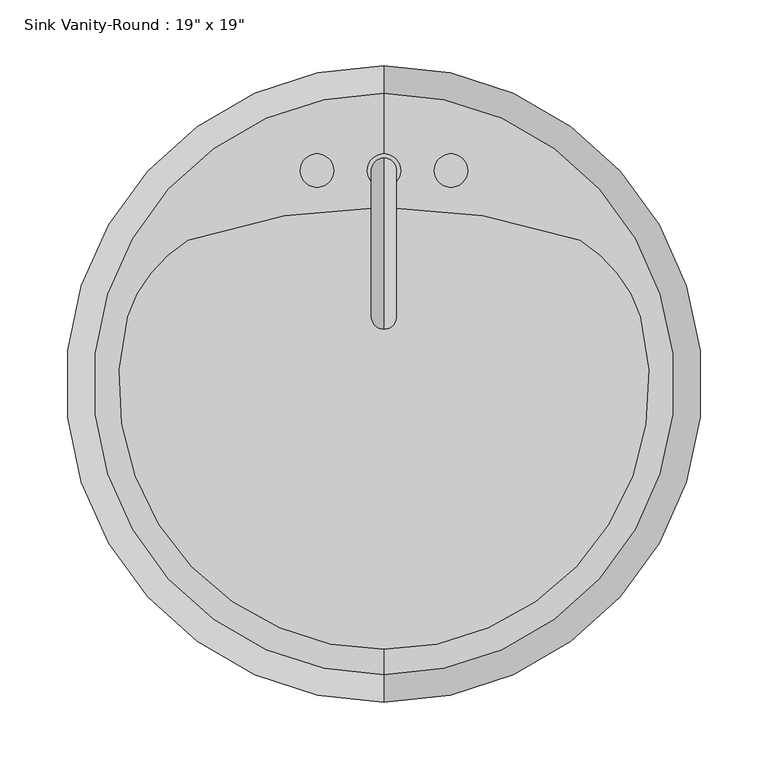
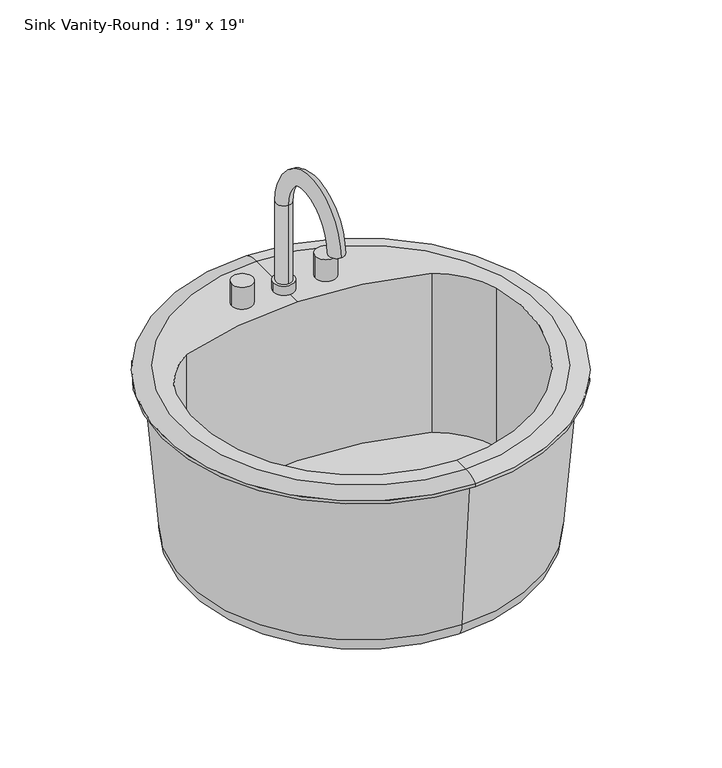
"""IFC4 building model written with IfcOpenShell, lengths in millimetres: flow terminal geometry."""

from ifc_helpers import new_model, si_unit, point, frame, frame_2d, origin, place, context, project, spatial, polyline, circle_curve, ellipse_curve, trimmed, segment, composite_curve, outline, extrude, source, transform, mapped, element, save
from ifc_brep_helpers import plane_surface, cylinder_surface, revolved_surface, advanced_brep


def flow_terminal_a43f4bde(model_context):
    return source(origin(), model_context, "Body", "SolidModel", [
        advanced_brep(
        [(96.6517406, -135.3870093, 796.925), (96.6517406, 305.7224463, 796.925), (96.6517406, 326.4677185, 791.36875), (96.6517406, -156.1322815, 791.36875), (96.6517406, -116.2405705, 796.925), (-98.1703414, 136.2525038, 796.925), (-52.1534933, 194.0861398, 796.925), (96.6517406, 219.2662048, 796.925), (245.4569744, 194.0861398, 796.925), (291.4738225, 136.2525038, 796.925), (96.6517406, -107.1264028, 571.5), (96.6517406, 277.4618398, 571.5), (96.6517406, 85.1677185, 571.5), (96.6517406, -127.6827361, 592.6842611), (96.6517406, 298.0181731, 592.6842611), (96.6517406, -144.2260315, 787.4), (96.6517406, 314.5614685, 787.4), (96.6517406, -156.1322815, 787.4), (96.6517406, 326.4677185, 787.4), (245.4569744, 194.0861398, 592.6842611), (-52.1534933, 194.0861398, 592.6842611), (-98.1703414, 136.2525038, 592.6842611), (291.4738225, 136.2525038, 592.6842611)],
        [
            (0, 1, circle_curve(frame((96.6517406, 85.1677185, 796.925), z_axis=(0.0, 0.0, -1.0), x_axis=(0.0, 1.0, 0.0)), 220.5547278)),
            (1, 2, circle_curve(frame((96.6517406, 309.4374616, 769.289434), z_axis=(-1.0, 0.0, 0.0), x_axis=(0.0, 1.0, 0.0)), 27.8841505)),
            (2, 3, circle_curve(frame((96.6517406, 85.1677185, 791.36875), z_axis=(0.0, 0.0, 1.0), x_axis=(0.0, 1.0, 0.0)), 241.3)),
            (3, 0, circle_curve(frame((96.6517406, -139.1020246, 769.289434), z_axis=(-1.0, 0.0, 0.0), x_axis=(0.0, -1.0, 0.0)), 27.8841505)),
            (1, 0, circle_curve(frame((96.6517406, 85.1677185, 796.925), z_axis=(0.0, 0.0, -1.0), x_axis=(0.0, 1.0, 0.0)), 220.5547278)),
            (3, 2, circle_curve(frame((96.6517406, 85.1677185, 791.36875), z_axis=(0.0, 0.0, 1.0), x_axis=(0.0, 1.0, 0.0)), 241.3)),
            (0, 4),
            (4, 5, circle_curve(frame((96.6517406, 85.1677185, 796.925), z_axis=(0.0, 0.0, -1.0), x_axis=(1.0, 0.0, 0.0)), 201.408289)),
            (5, 6, circle_curve(frame((1.3689689, 104.2755165, 796.925), z_axis=(0.0, 0.0, -1.0), x_axis=(1.0, 0.0, 0.0)), 104.5495194)),
            (6, 7, circle_curve(frame((96.6517406, -233.0168462, 796.925), z_axis=(0.0, 0.0, -1.0), x_axis=(1.0, 0.0, 0.0)), 452.283051)),
            (7, 1),
            (7, 8, circle_curve(frame((96.6517406, -233.0168462, 796.925), z_axis=(0.0, 0.0, -1.0), x_axis=(1.0, 0.0, 0.0)), 452.283051)),
            (8, 9, circle_curve(frame((191.9345122, 104.2755165, 796.925), z_axis=(0.0, 0.0, -1.0), x_axis=(1.0, 0.0, 0.0)), 104.5495194)),
            (9, 4, circle_curve(frame((96.6517406, 85.1677185, 796.925), z_axis=(0.0, 0.0, -1.0), x_axis=(1.0, 0.0, 0.0)), 201.408289)),
            (10, 11, circle_curve(frame((96.6517406, 85.1677185, 571.5), z_axis=(0.0, 0.0, -1.0), x_axis=(0.0, 1.0, 0.0)), 192.2941213)),
            (11, 12),
            (12, 10),
            (11, 10, circle_curve(frame((96.6517406, 85.1677185, 571.5), z_axis=(0.0, 0.0, -1.0), x_axis=(0.0, 1.0, 0.0)), 192.2941213)),
            (10, 13, circle_curve(frame((96.6517406, -107.1264028, 592.0656396), z_axis=(-1.0, 0.0, 0.0), x_axis=(0.0, -1.0, 0.0)), 20.5656396)),
            (13, 14, circle_curve(frame((96.6517406, 85.1677185, 592.6842611), z_axis=(0.0, 0.0, -1.0), x_axis=(0.0, 1.0, 0.0)), 212.8504546)),
            (14, 11, circle_curve(frame((96.6517406, 277.4618398, 592.0656396), z_axis=(-1.0, 0.0, 0.0), x_axis=(0.0, 1.0, 0.0)), 20.5656396)),
            (14, 13, circle_curve(frame((96.6517406, 85.1677185, 592.6842611), z_axis=(0.0, 0.0, -1.0), x_axis=(0.0, 1.0, 0.0)), 212.8504546)),
            (13, 15),
            (15, 16, circle_curve(frame((96.6517406, 85.1677185, 787.4), z_axis=(0.0, 0.0, -1.0), x_axis=(0.0, 1.0, 0.0)), 229.39375)),
            (16, 14),
            (16, 15, circle_curve(frame((96.6517406, 85.1677185, 787.4), z_axis=(0.0, 0.0, -1.0), x_axis=(0.0, 1.0, 0.0)), 229.39375)),
            (15, 17),
            (17, 18, circle_curve(frame((96.6517406, 85.1677185, 787.4), z_axis=(0.0, 0.0, -1.0), x_axis=(0.0, 1.0, 0.0)), 241.3)),
            (18, 16),
            (18, 17, circle_curve(frame((96.6517406, 85.1677185, 787.4), z_axis=(0.0, 0.0, -1.0), x_axis=(0.0, 1.0, 0.0)), 241.3)),
            (2, 18),
            (17, 3),
            (19, 20, circle_curve(frame((96.6517406, -233.0168462, 592.6842611), z_axis=(0.0, 0.0, 1.0), x_axis=(1.0, 0.0, 0.0)), 452.283051)),
            (20, 21, circle_curve(frame((1.3689689, 104.2755165, 592.6842611), z_axis=(0.0, 0.0, 1.0), x_axis=(1.0, 0.0, 0.0)), 104.5495194)),
            (21, 22, circle_curve(frame((96.6517406, 85.1677185, 592.6842611), z_axis=(0.0, 0.0, 1.0), x_axis=(1.0, 0.0, 0.0)), 201.408289)),
            (22, 19, circle_curve(frame((191.9345122, 104.2755165, 592.6842611), z_axis=(0.0, 0.0, 1.0), x_axis=(1.0, 0.0, 0.0)), 104.5495194)),
            (19, 8),
            (6, 20),
            (5, 21),
            (9, 22),
        ],
        [
            revolved_surface(trimmed(ellipse_curve(frame((96.6517406, 309.4374616, 769.289434), z_axis=(1.0, 0.0, 0.0), x_axis=(0.0, 1.0, 0.0)), 27.8841505, 27.8841505), [point((96.6517406, 326.4677185, 791.36875))], [point((96.6517406, 305.7224463, 796.925))], True, "CARTESIAN"), (96.6517406, 85.1677185, 796.925), (0.0, 0.0, 1.0)),
            plane_surface(frame((96.6517406, 85.1677185, 796.925), z_axis=(0.0, 0.0, 1.0), x_axis=(0.0, 1.0, 0.0))),
            plane_surface(frame((96.6517406, 85.1677185, 571.5), z_axis=(0.0, 0.0, -1.0), x_axis=(0.0, 1.0, 0.0))),
            revolved_surface(trimmed(ellipse_curve(frame((96.6517406, 277.4618398, 592.0656396), z_axis=(1.0, 0.0, 0.0), x_axis=(0.0, 1.0, 0.0)), 20.5656396, 20.5656396), [point((96.6517406, 277.4618398, 571.5))], [point((96.6517406, 298.0181731, 592.6842611))], True, "CARTESIAN"), (96.6517406, 85.1677185, 796.925), (0.0, 0.0, 1.0)),
            revolved_surface(polyline([(96.6517406, 298.0181731, 592.6842611), (96.6517406, 314.5614685, 787.4)]), (96.6517406, 85.1677185, 796.925), (0.0, 0.0, 1.0)),
            plane_surface(frame((96.6517406, 85.1677185, 787.4), z_axis=(0.0, 0.0, -1.0), x_axis=(0.0, 1.0, 0.0))),
            cylinder_surface(frame((96.6517406, 85.1677185, 796.925), z_axis=(0.0, 0.0, 1.0), x_axis=(0.0, 1.0, 0.0)), 241.3),
            plane_surface(frame((548.9347916, -233.0168462, 592.6842611), z_axis=(0.0, 0.0, 1.0), x_axis=(0.0, -1.0, 0.0))),
            revolved_surface(polyline([(548.9347916, -233.0168462, 796.925), (548.9347916, -233.0168462, 592.6842611)]), (96.6517406, -233.0168462, 592.6842611), (0.0, 0.0, 1.0)),
            revolved_surface(polyline([(105.91848829999999, 104.2755165, 796.925), (105.91848829999999, 104.2755165, 592.6842611)]), (1.3689689, 104.2755165, 592.6842611), (0.0, 0.0, 1.0)),
            revolved_surface(polyline([(298.0600296, 85.1677185, 796.925), (298.0600296, 85.1677185, 592.6842611)]), (96.6517406, 85.1677185, 592.6842611), (0.0, 0.0, 1.0)),
            revolved_surface(polyline([(296.4840316, 104.2755165, 796.925), (296.4840316, 104.2755165, 592.6842611)]), (191.9345122, 104.2755165, 592.6842611), (0.0, 0.0, 1.0)),
        ],
        [
            (0, [[1, 2, 3, 4]]),
            (0, [[-2, 5, -4, 6]]),
            (1, [[-1, 7, 8, 9, 10, 11]]),
            (1, [[-5, -11, 12, 13, 14, -7]]),
            (2, [[15, 16, 17]]),
            (2, [[-16, 18, -17]]),
            (3, [[-15, 19, 20, 21]]),
            (3, [[-18, -21, 22, -19]]),
            (4, [[-20, 23, 24, 25]]),
            (4, [[-22, -25, 26, -23]]),
            (5, [[-24, 27, 28, 29]]),
            (5, [[-26, -29, 30, -27]]),
            (6, [[-3, 31, -28, 32]]),
            (6, [[-6, -32, -30, -31]]),
            (7, [[33, 34, 35, 36]]),
            (8, [[-33, 37, -12, -10, 38]]),
            (9, [[-34, -38, -9, 39]]),
            (10, [[-35, -39, -8, -14, 40]]),
            (11, [[-36, -40, -13, -37]]),
        ],
    ),
        extrude(outline(composite_curve([segment(trimmed(circle_curve(frame_2d((96.6517406, 85.1677185)), 20.6375), [point((76.0142406, 85.1677185))], [point((117.2892406, 85.1677185))], False, "CARTESIAN"), True, "CONTINUOUS"), segment(trimmed(circle_curve(frame_2d((96.6517406, 85.1677185)), 20.6375), [point((117.2892406, 85.1677185))], [point((76.0142406, 85.1677185))], False, "CARTESIAN"), True, "CONTINUOUS")], self_intersect=False)), frame((0.0, 0.0, 571.5), z_axis=(0.0, 0.0, 1.0), x_axis=(1.0, 0.0, 0.0)), (0.0, 0.0, 1.0), 21.1842611),
        extrude(outline(composite_curve([segment(trimmed(circle_curve(frame_2d((147.4517406, 247.0927185)), 12.7), [point((134.7517406, 247.0927185))], [point((160.1517406, 247.0927185))], False, "CARTESIAN"), True, "CONTINUOUS"), segment(trimmed(circle_curve(frame_2d((147.4517406, 247.0927185)), 12.7), [point((160.1517406, 247.0927185))], [point((134.7517406, 247.0927185))], False, "CARTESIAN"), True, "CONTINUOUS")], self_intersect=False)), frame((0.0, 0.0, 796.925), z_axis=(0.0, 0.0, 1.0), x_axis=(1.0, 0.0, 0.0)), (0.0, 0.0, 1.0), 28.575),
        extrude(outline(composite_curve([segment(trimmed(circle_curve(frame_2d((45.8517406, 247.0927185)), 12.7), [point((33.1517406, 247.0927185))], [point((58.5517406, 247.0927185))], False, "CARTESIAN"), True, "CONTINUOUS"), segment(trimmed(circle_curve(frame_2d((45.8517406, 247.0927185)), 12.7), [point((58.5517406, 247.0927185))], [point((33.1517406, 247.0927185))], False, "CARTESIAN"), True, "CONTINUOUS")], self_intersect=False)), frame((0.0, 0.0, 796.925), z_axis=(0.0, 0.0, 1.0), x_axis=(1.0, 0.0, 0.0)), (0.0, 0.0, 1.0), 28.575),
        advanced_brep(
        [(83.9517406, 247.0927185, 796.925), (109.3517406, 247.0927185, 796.925), (96.6517406, 237.5677185, 909.6375), (96.6517406, 256.6177185, 909.6375), (96.6517406, 256.6177185, 809.1602909), (96.6517406, 237.5677185, 809.1602909), (96.6517406, 145.7775038, 909.6375), (96.6517406, 126.7275038, 909.6375), (83.9517406, 247.0927185, 809.1602909), (109.3517406, 247.0927185, 809.1602909)],
        [
            (0, 1, circle_curve(frame((96.6517406, 247.0927185, 796.925), z_axis=(0.0, 0.0, -1.0), x_axis=(1.0, 0.0, 0.0)), 12.7)),
            (1, 0, circle_curve(frame((96.6517406, 247.0927185, 796.925), z_axis=(0.0, 0.0, -1.0), x_axis=(1.0, 0.0, 0.0)), 12.7)),
            (2, 3, circle_curve(frame((96.6517406, 247.0927185, 909.6375), z_axis=(0.0, 0.0, -1.0), x_axis=(0.0, 1.0, 0.0)), 9.525)),
            (3, 4),
            (4, 5, circle_curve(frame((96.6517406, 247.0927185, 809.1602909), z_axis=(0.0, 0.0, 1.0), x_axis=(0.0, 1.0, 0.0)), 9.525)),
            (5, 2),
            (3, 2, circle_curve(frame((96.6517406, 247.0927185, 909.6375), z_axis=(0.0, 0.0, -1.0), x_axis=(0.0, 1.0, 0.0)), 9.525)),
            (5, 4, circle_curve(frame((96.6517406, 247.0927185, 809.1602909), z_axis=(0.0, 0.0, 1.0), x_axis=(0.0, 1.0, 0.0)), 9.525)),
            (6, 7, circle_curve(frame((96.6517406, 136.2525038, 909.6375), z_axis=(0.0, 0.0, -1.0), x_axis=(0.0, -1.0, 0.0)), 9.525)),
            (7, 6, circle_curve(frame((96.6517406, 136.2525038, 909.6375), z_axis=(0.0, 0.0, -1.0), x_axis=(0.0, -1.0, 0.0)), 9.525)),
            (2, 6, circle_curve(frame((96.6517406, 191.6726112, 909.6375), z_axis=(1.0, 0.0, 0.0), x_axis=(0.0, 1.0, 0.0)), 45.8951073)),
            (7, 3, circle_curve(frame((96.6517406, 191.6726112, 909.6375), z_axis=(-1.0, 0.0, 0.0), x_axis=(0.0, 1.0, 0.0)), 64.9451073)),
            (8, 9, circle_curve(frame((96.6517406, 247.0927185, 809.1602909), z_axis=(0.0, 0.0, 1.0), x_axis=(1.0, 0.0, 0.0)), 12.7)),
            (9, 8, circle_curve(frame((96.6517406, 247.0927185, 809.1602909), z_axis=(0.0, 0.0, 1.0), x_axis=(1.0, 0.0, 0.0)), 12.7)),
            (8, 0),
            (1, 9),
        ],
        [
            plane_surface(frame((96.6517406, 237.5677185, 796.925), z_axis=(0.0, 0.0, -1.0), x_axis=(1.0, 0.0, 0.0))),
            cylinder_surface(frame((96.6517406, 247.0927185, 796.925), z_axis=(0.0, 0.0, -1.0), x_axis=(0.0, 1.0, 0.0)), 9.525),
            plane_surface(frame((96.6517406, 191.6726112, 909.6375), z_axis=(0.0, 0.0, -1.0), x_axis=(0.0, -1.0, 0.0))),
            revolved_surface(trimmed(ellipse_curve(frame((96.6517406, 247.0927185, 909.6375), z_axis=(0.0, 0.0, -1.0), x_axis=(0.0, 1.0, 0.0)), 9.525, 9.525), [point((96.6517406, 237.5677185, 909.6375))], [point((96.6517406, 256.6177185, 909.6375))], True, "CARTESIAN"), (96.6517406, 191.6726112, 909.6375), (1.0, 0.0, 0.0)),
            revolved_surface(trimmed(ellipse_curve(frame((96.6517406, 247.0927185, 909.6375), z_axis=(0.0, 0.0, -1.0), x_axis=(0.0, 1.0, 0.0)), 9.525, 9.525), [point((96.6517406, 256.6177185, 909.6375))], [point((96.6517406, 237.5677185, 909.6375))], True, "CARTESIAN"), (96.6517406, 191.6726112, 909.6375), (1.0, 0.0, 0.0)),
            plane_surface(frame((109.3517406, 247.0927185, 809.1602909), z_axis=(0.0, 0.0, 1.0), x_axis=(0.0, 1.0, 0.0))),
            cylinder_surface(frame((96.6517406, 247.0927185, 796.925), z_axis=(0.0, 0.0, 1.0), x_axis=(1.0, 0.0, 0.0)), 12.7),
        ],
        [
            (0, [[1, 2]]),
            (1, [[3, 4, 5, 6]]),
            (1, [[7, -6, 8, -4]]),
            (2, [[9, 10]]),
            (3, [[-3, 11, -10, 12]]),
            (4, [[-7, -12, -9, -11]]),
            (5, [[13, 14], [-5, -8]]),
            (6, [[-13, 15, -2, 16]]),
            (6, [[-14, -16, -1, -15]]),
        ],
    ),
    ])


if __name__ == "__main__":
    model = new_model("IFC4")
    model_context = context("Model", 3, world=origin())
    ifc_project = project(units=[si_unit("LENGTHUNIT", "METRE", prefix="MILLI")], contexts=[model_context])
    site = spatial("IfcSite", under=ifc_project)
    building = spatial("IfcBuilding", under=site)
    placement = place(None, origin())
    flow_terminal_shape = flow_terminal_a43f4bde(model_context)
    element("IfcFlowTerminal", 1, ObjectType="Sink Vanity-Round : 19\" x 19\"", at=placement, inside=building, context=model_context, shape_type="MappedRepresentation", body=[
        mapped(flow_terminal_shape, transform((0.0, 0.0, 0.0), x_axis=(1.0, 0.0, 0.0), y_axis=(0.0, 1.0, 0.0), z_axis=(0.0, 0.0, 1.0))),
    ])
    save(model, "model.ifc")

# Revit data of these elements
# Type "Sink Vanity-Round : 19\" x 19\""
#   Assembly Code = "D2010400"
#   Top Of Counter = 2' - 7"
#   Basin Material = Porcelain, Linen
#   Faucet Material = Steel, Polished
#   Default Elevation = 0
# Element 1 (IfcFlowTerminal, "Sink Vanity-Round : 19\" x 19\"")
#   Materials on its faces: "Porcelain, Linen", "Steel, Polished"
# Materials
#   "Porcelain, Linen": class "Ceramic", colour RGB 249 239 230, transparency 0, Description = "Porcelain, linen", Cost = 0
#   "Steel, Polished": class "Metal", colour RGB 57 57 57, transparency 0, Description = "Polished steel", Cost = 0
